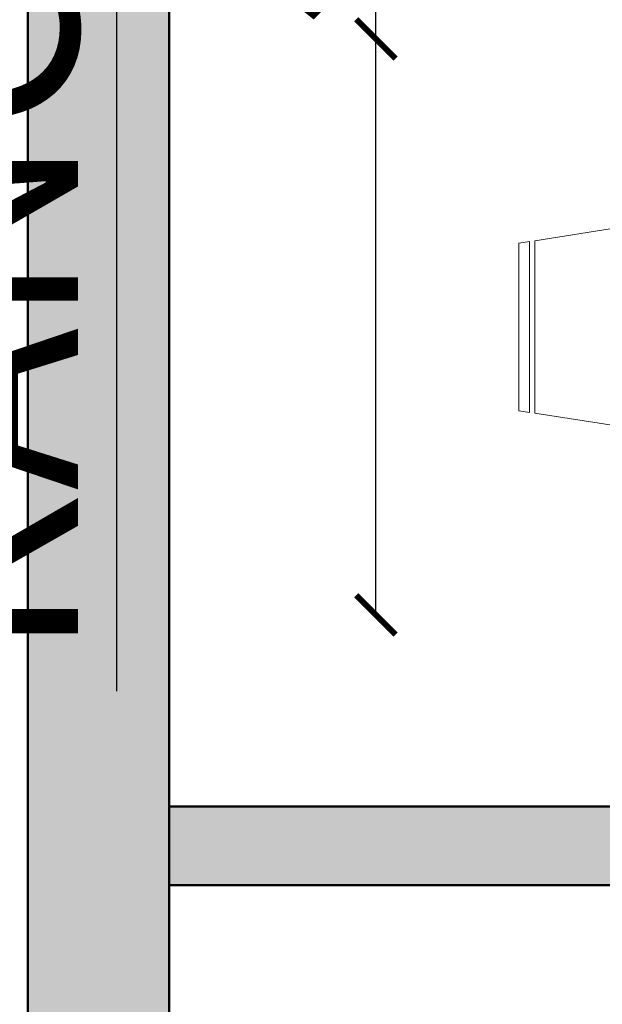
# Model space of a CAD drawing. Units: inches. Extents: x 2419 to 2878, y 1068 to 1713.
# Tile 3 of 20: x 2471 to 2508, y 1286 to 1349. Entities that reach past the tile are written whole.
import ezdxf

# ---------------------------------------------------------------- set-up
doc = ezdxf.new("R2010")
doc.units = ezdxf.units.IN
for name, color, linetype, lineweight in [('A-ANNO-DIMS', 2, 'Continuous', 18), ('A-FLOR-PRKG-PATT', 1, 'Continuous', 13), ('A-FURN', 8, 'Continuous', 18), ('A-WALL', 7, 'Continuous', 50)]:
    doc.layers.add(name, color=color, linetype=linetype, lineweight=lineweight)
doc.layers.add('A-WALL-PATT', color=18, linetype='Continuous', lineweight=13, true_color=0x000000)
doc.styles.get("Standard").update_dxf_attribs({"font": 'arial.ttf'})
doc.dimstyles.new('ISO-25', dxfattribs={"dimtxt": 12.5, "dimasz": 2.5, "dimexe": 1.25, "dimexo": 0.625, "dimtad": 1, "dimdec": 0, "dimlunit": 4, "dimtxsty": 'Standard', "dimblk": 'ARCHTICK', "dimcen": 2.5, "dimse1": 1, "dimse2": 1, "dimclrd": 4, "dimadec": 0, "dimazin": 0, "dimtfac": 1, "dimtdec": 0, "dimtmove": 0, "dimatfit": 3, "dimfxl": 1, "dimarcsym": 0})

# ---------------------------------------------------------------- blocks, each defined once
blk = doc.blocks.new('Dining Set - 36 x 72 in.')
for p, q in [((-22, 27.5), (-22.1562, 26.50042)), ((-22, 27.5), (-6, 27.5)), ((-5.8437, 26.49966), (-6, 27.5)), ((6, 27.5), (5.8438, 26.50042)), ((6, 27.5), (22, 27.5)), ((22.1563, 26.49966), (22, 27.5)), ((-5.8416, 26.5), (-22.1534, 26.5)), ((22.1584, 26.5), (5.8466, 26.5)), ((-22.2343, 26.00059), (-23.4847, 17.99762)), ((-22.2304, 26), (-5.7608, 26)), ((-4.5152, 17.99762), (-5.7655, 25.99926)), ((5.7657, 26.00059), (4.5153, 17.99762)), ((5.7696, 26), (22.2392, 26)), ((23.4848, 17.99762), (22.2345, 25.99926)), ((36, 18), (-36, 18)), ((-36, 18), (-36, -18)), ((36, -18), (36, 18)), ((-44.0006, 8.23428), (-35.9976, 9.48474)), ((44.0006, 8.23428), (35.9976, 9.48474)), ((-45.5, 8), (-44.5004, 8.15617)), ((-45.5, 8), (-45.5, -8)), ((-44.5, -8.15843), (-44.5, 8.15338)), ((-44, 8.23041), (-44, -8.23915)), ((44, 8.23041), (44, -8.23915)), ((44.5, -8.15843), (44.5, 8.15338)), ((45.5, 8), (44.5005, 8.15617)), ((45.5, 8), (45.5, -8)), ((-44.4997, -8.15631), (-45.5, -8)), ((-35.9976, -9.48476), (-43.9993, -8.2345)), ((35.9976, -9.48476), (43.9993, -8.2345)), ((44.4997, -8.15631), (45.5, -8)), ((-36, -18), (36, -18)), ((-22.2343, -26.0006), (-23.4847, -17.99762)), ((-4.5152, -17.99762), (-5.7655, -25.99928)), ((5.7657, -26.0006), (4.5153, -17.99762)), ((23.4848, -17.99762), (22.2345, -25.99928)), ((-22.2304, -26), (-5.7608, -26)), ((5.7696, -26), (22.2392, -26)), ((-22, -27.5), (-22.1562, -26.50044)), ((-5.8416, -26.5), (-22.1534, -26.5)), ((-5.8437, -26.49967), (-6, -27.5)), ((6, -27.5), (5.8438, -26.50044)), ((22.1584, -26.5), (5.8466, -26.5)), ((22.1563, -26.49967), (22, -27.5)), ((-22, -27.5), (-6, -27.5)), ((6, -27.5), (22, -27.5))]:
    blk.add_line(p, q)
for points in [[(-36, 15), (-31.1772, 14.97754), (-26.8079, 14.91406), (-22.8538, 14.81543), (-19.276, 14.6875), (-16.0362, 14.53613), (-13.0957, 14.36718), (-10.4159, 14.18652), (-7.9583, 14), (-5.6904, 13.81315), (-3.6035, 13.63021), (-1.6954, 13.45508), (0.0365, 13.29166), (1.5945, 13.14388), (2.9811, 13.01562), (4.1988, 12.9108), (5.25, 12.83333), (6.1393, 12.78613), (6.8802, 12.76823), (7.4883, 12.77767), (7.9792, 12.8125), (8.3685, 12.87077), (8.6719, 12.95052), (8.9049, 13.0498), (9.0833, 13.16666), (9.2205, 13.29899), (9.3216, 13.44401), (9.3895, 13.59879), (9.4271, 13.76041), (9.4373, 13.92594), (9.4232, 14.09245), (9.3875, 14.257), (9.3333, 14.41666), (9.2638, 14.56917), (9.1836, 14.71484), (9.0975, 14.85465), (9.0104, 14.98958), (8.9272, 15.1206), (8.8529, 15.2487), (8.7922, 15.37483), (8.75, 15.5), (8.7305, 15.62467), (8.7344, 15.74739), (8.7617, 15.86621), (8.8125, 15.97916), (8.8867, 16.08431), (8.9844, 16.17968), (9.1055, 16.26334), (9.25, 16.33333), (9.4189, 16.38802), (9.6172, 16.42708), (9.8506, 16.45052), (10.125, 16.45833), (10.4463, 16.45052), (10.8203, 16.42708), (11.2529, 16.38802), (11.75, 16.33333), (12.3184, 16.26318), (12.9694, 16.17838), (13.7151, 16.07991), (14.5677, 15.96875), (15.5395, 15.84586), (16.6426, 15.71224), (17.8893, 15.56884), (19.2917, 15.41666), (20.859, 15.25667), (22.5879, 15.08984), (24.4721, 14.91715), (26.5052, 14.73958), (28.6809, 14.5581), (30.9929, 14.3737), (33.4347, 14.18733), (36, 14)], [(-36, 10), (-28.9766, 10.14274), (-23.1725, 10.20442), (-18.4241, 10.19775), (-14.5677, 10.13541), (-11.4399, 10.03011), (-8.877, 9.89453), (-6.7154, 9.74137), (-4.7917, 9.58333), (-2.9698, 9.43082), (-1.2246, 9.28515), (0.4415, 9.14534), (2.026, 9.01041), (3.5266, 8.87939), (4.9408, 8.7513), (6.266, 8.62516), (7.5, 8.5), (8.6411, 8.37549), (9.6914, 8.2539), (10.6538, 8.13818), (11.5312, 8.03125), (12.3267, 7.93603), (13.043, 7.85547), (13.6831, 7.79248), (14.25, 7.75), (14.7471, 7.7303), (15.1797, 7.73307), (15.5537, 7.75732), (15.875, 7.80208), (16.1494, 7.86637), (16.3828, 7.94922), (16.5811, 8.04964), (16.75, 8.16666), (16.8944, 8.29915), (17.0143, 8.44531), (17.1089, 8.60319), (17.1771, 8.77083), (17.218, 8.94629), (17.2305, 9.1276), (17.2137, 9.31282), (17.1667, 9.5), (17.0895, 9.6875), (16.987, 9.875), (16.8649, 10.0625), (16.7292, 10.25), (16.5856, 10.4375), (16.4401, 10.625), (16.2985, 10.8125), (16.1667, 11), (16.05, 11.18733), (15.9518, 11.3737), (15.8752, 11.5581), (15.8229, 11.73958), (15.798, 11.91715), (15.8034, 12.08984), (15.842, 12.25667), (15.9167, 12.41666), (16.0295, 12.56836), (16.1784, 12.70833), (16.3605, 12.83268), (16.5729, 12.9375), (16.8127, 13.01888), (17.0768, 13.07291), (17.3625, 13.0957), (17.6667, 13.08333), (17.9894, 13.03312), (18.3418, 12.94726), (18.7382, 12.82918), (19.1927, 12.68229), (19.7195, 12.51001), (20.3327, 12.31575), (21.0465, 12.10294), (21.875, 11.875), (22.8357, 11.63354), (23.959, 11.37304), (25.2786, 11.08618), (26.8282, 10.76562), (28.6414, 10.40405), (30.752, 9.99414), (33.1936, 9.52856), (36, 9)], [(-36, 5.5), (-30.7157, 5.3348), (-26.069, 5.20963), (-21.9946, 5.11767), (-18.4271, 5.05208), (-15.3009, 5.00602), (-12.5508, 4.97265), (-10.1112, 4.94515), (-7.9167, 4.91666), (-5.909, 4.88167), (-4.0586, 4.83984), (-2.3429, 4.79215), (-0.7396, 4.73958), (0.7739, 4.6831), (2.22, 4.6237), (3.6213, 4.56233), (5, 4.5), (6.373, 4.43782), (7.7344, 4.3776), (9.0723, 4.32129), (10.375, 4.27083), (11.6309, 4.22819), (12.8281, 4.19531), (13.9551, 4.17415), (15, 4.16666), (15.954, 4.17448), (16.819, 4.19791), (17.6001, 4.23698), (18.3021, 4.29166), (18.9299, 4.36198), (19.4883, 4.44791), (19.9823, 4.54948), (20.4167, 4.66666), (20.7969, 4.79899), (21.1302, 4.94401), (21.4245, 5.09879), (21.6875, 5.26041), (21.9271, 5.42594), (22.1511, 5.59245), (22.3672, 5.757), (22.5834, 5.91666), (22.8065, 6.06868), (23.0404, 6.21093), (23.2879, 6.34147), (23.5521, 6.45833), (23.8358, 6.55957), (24.142, 6.64323), (24.4735, 6.70735), (24.8334, 6.75), (25.2235, 6.76969), (25.642, 6.76692), (26.0858, 6.74267), (26.5521, 6.69791), (27.0379, 6.63362), (27.5404, 6.55078), (28.0565, 6.45036), (28.5834, 6.33333), (29.1242, 6.19987), (29.7071, 6.04687), (30.3661, 5.87044), (31.1354, 5.66666), (32.0493, 5.43164), (33.142, 5.16146), (34.4475, 4.85221), (36, 4.5)], [(-36, -1), (-30.7915, -0.6591), (-26.0195, -0.38216), (-21.6519, -0.16284), (-17.6563, 0.00521), (-14.0005, 0.12833), (-10.6523, 0.21289), (-7.5796, 0.26522), (-4.75, 0.29166), (-2.134, 0.29793), (0.2878, 0.28711), (2.5317, 0.26163), (4.6146, 0.22396), (6.5529, 0.17651), (8.3633, 0.12174), (10.0623, 0.06209), (11.6667, 0), (13.1899, -0.06201), (14.6341, -0.1211), (15.9982, -0.17432), (17.2813, -0.21875), (18.4823, -0.25147), (19.6003, -0.26953), (20.6343, -0.27002), (21.5834, -0.25), (22.4481, -0.20768), (23.2357, -0.14584), (23.9549, -0.06836), (24.6146, 0.02083), (25.2235, 0.11784), (25.7904, 0.21875), (26.3241, 0.31966), (26.8334, 0.41666), (27.3265, 0.50618), (27.8099, 0.58593), (28.2894, 0.65397), (28.7709, 0.70833), (29.2601, 0.74707), (29.763, 0.76823), (30.2855, 0.76985), (30.8334, 0.75), (31.4088, 0.70784), (31.9994, 0.64713), (32.589, 0.57275), (33.1615, 0.48958), (33.7008, 0.4025), (34.1908, 0.3164), (34.6153, 0.23616), (34.9584, 0.16666), (35.2099, 0.11165), (35.3848, 0.07031), (35.504, 0.04069), (35.5886, 0.02083), (35.6594, 0.00879), (35.7377, 0.0026), (35.8442, 0.00032), (36, 0)], [(-36, -6.5), (-27.1843, -6.31267), (-20.084, -6.1263), (-14.469, -5.9419), (-10.1094, -5.76042), (-6.7752, -5.58285), (-4.2363, -5.41016), (-2.2629, -5.24333), (-0.625, -5.08334), (0.8708, -4.93099), (2.2715, -4.78646), (3.5872, -4.64974), (4.8281, -4.52084), (6.0046, -4.39974), (7.127, -4.28646), (8.2053, -4.18099), (9.25, -4.08334), (10.2705, -3.99382), (11.2734, -3.91407), (12.2647, -3.84603), (13.25, -3.79167), (14.2354, -3.75293), (15.2266, -3.73177), (16.2295, -3.73015), (17.25, -3.75), (18.2912, -3.79248), (19.3451, -3.85547), (20.4009, -3.93604), (21.4479, -4.03125), (22.4754, -4.13819), (23.4727, -4.25391), (24.4289, -4.37549), (25.3334, -4.5), (26.1785, -4.62492), (26.9694, -4.74935), (27.7145, -4.87281), (28.4219, -4.99479), (29.1, -5.11483), (29.7572, -5.23242), (30.4016, -5.34709), (31.0417, -5.45834), (31.6837, -5.56437), (32.3262, -5.65821), (32.9658, -5.73153), (33.599, -5.77604), (34.2224, -5.78345), (34.8327, -5.74545), (35.4264, -5.65373), (36, -5.5)], [(-36, -10), (-26.4022, -9.81299), (-18.4675, -9.62891), (-11.9839, -9.45069), (-6.7396, -9.28125), (-2.5226, -9.12354), (0.8789, -8.98047), (3.6769, -8.85498), (6.0833, -8.75), (8.2767, -8.66765), (10.3021, -8.60677), (12.1712, -8.56543), (13.8958, -8.54167), (15.4876, -8.53353), (16.9583, -8.53907), (18.3197, -8.55632), (19.5834, -8.58334), (20.7616, -8.61841), (21.8685, -8.66081), (22.9188, -8.71004), (23.9271, -8.76563), (24.9081, -8.82707), (25.8763, -8.89388), (26.8465, -8.96558), (27.8334, -9.04167), (28.8474, -9.12118), (29.8828, -9.20117), (30.93, -9.27824), (31.9792, -9.34896), (33.0205, -9.40991), (34.0443, -9.45768), (35.0407, -9.48885), (36, -9.5)], [(-36, -14.5), (-30.0881, -14.33513), (-25.0332, -14.21224), (-20.7312, -14.12647), (-17.0781, -14.07292), (-13.97, -14.04671), (-11.3027, -14.04297), (-8.9724, -14.05681), (-6.875, -14.08334), (-4.9224, -14.11833), (-3.0905, -14.16016), (-1.3709, -14.20785), (0.2448, -14.26042), (1.7647, -14.3169), (3.1973, -14.3763), (4.5507, -14.43767), (5.8333, -14.5), (7.0554, -14.5621), (8.235, -14.62175), (9.3922, -14.67652), (10.5469, -14.72396), (11.7192, -14.76164), (12.929, -14.78711), (14.1965, -14.79794), (15.5417, -14.79167), (16.9933, -14.76424), (18.6152, -14.70508), (20.4804, -14.60197), (22.6615, -14.44271), (25.2312, -14.21509), (28.2624, -13.9069), (31.8277, -13.50594), (36, -13)]]:
    blk.add_lwpolyline(points)
blk = doc.blocks.new('_ArchTick')
at = {"color": 0, "linetype": 'ByBlock', "const_width": 0.15}
blk.add_lwpolyline([(-0.5, -0.5), (0.5, 0.5)], dxfattribs=at)
blk = doc.blocks.new('*D26')
at = {"layer": 'A-ANNO-DIMS', "color": 4, "lineweight": -2, "transparency": 16777216}
for p, q in [((2502.769, 1356.79), (2563.458, 1356.79)), ((2563.458, 1356.79), (2733.724, 1356.79))]:
    blk.add_line(p, q, dxfattribs=at)
at = {"layer": 'Defpoints', "color": 0, "transparency": 16777216}
for p in [(2563.458, 1356.79), (2502.769, 1347.687), (2563.458, 1347.687)]:
    blk.add_point(p, dxfattribs=at)
at = {"layer": 'A-ANNO-DIMS', "color": 4, "lineweight": -2, "transparency": 16777216, "xscale": 2.5, "yscale": 2.5, "zscale": 2.5, "rotation": 180}
blk.add_blockref('_ArchTick', (2502.769, 1356.79), dxfattribs=at)
at = {"layer": 'A-ANNO-DIMS', "color": 4, "lineweight": -2, "transparency": 16777216, "xscale": 2.5, "yscale": 2.5, "zscale": 2.5}
blk.add_blockref('_ArchTick', (2563.458, 1356.79), dxfattribs=at)
at = {"layer": 'A-ANNO-DIMS', "color": 0, "transparency": 16777216, "insert": (2649.841, 1363.878), "char_height": 12.5, "attachment_point": 5}
blk.add_mtext('DINING SET 5\'-0 1/2"', dxfattribs=at)
blk = doc.blocks.new('*D27')
at = {"layer": 'A-ANNO-DIMS', "color": 4, "lineweight": -2, "transparency": 16777216}
for p, q in [((2493.665, 1347.687), (2493.665, 1413.783)), ((2493.665, 1311.006), (2493.665, 1347.687))]:
    blk.add_line(p, q, dxfattribs=at)
at = {"layer": 'Defpoints', "color": 0, "transparency": 16777216}
for p in [(2493.665, 1347.687), (2502.769, 1347.687), (2502.769, 1311.006)]:
    blk.add_point(p, dxfattribs=at)
at = {"layer": 'A-ANNO-DIMS', "color": 4, "lineweight": -2, "transparency": 16777216, "xscale": 2.5, "yscale": 2.5, "zscale": 2.5}
for p, rotation in [((2493.665, 1347.687), 90), ((2493.665, 1311.006), 270)]:
    blk.add_blockref('_ArchTick', p, dxfattribs=dict(at, rotation=rotation))
at = {"layer": 'A-ANNO-DIMS', "color": 0, "transparency": 16777216, "insert": (2486.573, 1381.985), "char_height": 12.5, "attachment_point": 5, "rotation": 90}
blk.add_mtext('3\'-0 1/2"', dxfattribs=at)
blk = doc.blocks.new('*D28')
at = {"layer": 'A-ANNO-DIMS', "color": 4, "lineweight": -2, "transparency": 16777216}
for p, q in [((2477.16, 1470.633), (2477.16, 1448.272)), ((2477.16, 1448.272), (2477.16, 1306.152))]:
    blk.add_line(p, q, dxfattribs=at)
at = {"layer": 'Defpoints', "color": 0, "transparency": 16777216}
for p in [(2480.514, 1470.633), (2477.16, 1448.272), (2480.514, 1448.272)]:
    blk.add_point(p, dxfattribs=at)
at = {"layer": 'A-ANNO-DIMS', "color": 4, "lineweight": -2, "transparency": 16777216, "xscale": 2.5, "yscale": 2.5, "zscale": 2.5}
for p, rotation in [((2477.16, 1470.633), 90), ((2477.16, 1448.272), 270)]:
    blk.add_blockref('_ArchTick', p, dxfattribs=dict(at, rotation=rotation))
at = {"layer": 'A-ANNO-DIMS', "color": 0, "transparency": 16777216, "insert": (2470.072, 1375.962), "char_height": 12.5, "attachment_point": 5, "rotation": 90}
blk.add_mtext('RANGE 1\'-10 1/2"', dxfattribs=at)
blk = doc.blocks.new('*D43')
at = {"layer": 'A-ANNO-DIMS', "color": 4, "lineweight": -2, "transparency": 16777216}
blk.add_line((2480.514, 1079.925), (2557.299, 1079.925), dxfattribs=at)
at = {"layer": 'Defpoints', "color": 0, "transparency": 16777216}
for p in [(2480.514, 1408.813), (2557.299, 1408.813), (2557.299, 1079.925)]:
    blk.add_point(p, dxfattribs=at)
at = {"layer": 'A-ANNO-DIMS', "color": 4, "lineweight": -2, "transparency": 16777216, "xscale": 2.5, "yscale": 2.5, "zscale": 2.5, "rotation": 180}
blk.add_blockref('_ArchTick', (2480.514, 1079.925), dxfattribs=at)
at = {"layer": 'A-ANNO-DIMS', "color": 4, "lineweight": -2, "transparency": 16777216, "xscale": 2.5, "yscale": 2.5, "zscale": 2.5}
blk.add_blockref('_ArchTick', (2557.299, 1079.925), dxfattribs=at)
at = {"layer": 'A-ANNO-DIMS', "color": 0, "transparency": 16777216, "insert": (2518.907, 1086.932), "char_height": 12.5, "attachment_point": 5}
blk.add_mtext('6\'-5"', dxfattribs=at)
blk = doc.blocks.new('*D47')
at = {"layer": 'A-ANNO-DIMS', "color": 4, "lineweight": -2, "transparency": 16777216}
for p, q in [((2444.314, 1376.561), (2444.314, 1357.976)), ((2444.314, 1357.976), (2444.314, 1293.048))]:
    blk.add_line(p, q, dxfattribs=at)
at = {"layer": 'Defpoints', "color": 0, "transparency": 16777216}
for p in [(2632.514, 1376.561), (2444.314, 1357.976), (2632.514, 1357.976)]:
    blk.add_point(p, dxfattribs=at)
at = {"layer": 'A-ANNO-DIMS', "color": 4, "lineweight": -2, "transparency": 16777216, "xscale": 2.5, "yscale": 2.5, "zscale": 2.5}
for p, rotation in [((2444.314, 1376.561), 90), ((2444.314, 1357.976), 270)]:
    blk.add_blockref('_ArchTick', p, dxfattribs=dict(at, rotation=rotation))
at = {"layer": 'A-ANNO-DIMS', "color": 0, "transparency": 16777216, "insert": (2437.226, 1324.262), "char_height": 12.5, "attachment_point": 5, "rotation": 90}
blk.add_mtext('1\'-6 1/2"', dxfattribs=at)
blk = doc.blocks.new('*D54')
at = {"layer": 'A-ANNO-DIMS', "color": 4, "lineweight": -2, "transparency": 16777216}
blk.add_line((2444.314, 1130.813), (2444.314, 1293.813), dxfattribs=at)
at = {"layer": 'Defpoints', "color": 0, "transparency": 16777216}
for p in [(2444.314, 1293.813), (2480.514, 1293.813), (2480.514, 1130.813)]:
    blk.add_point(p, dxfattribs=at)
at = {"layer": 'A-ANNO-DIMS', "color": 4, "lineweight": -2, "transparency": 16777216, "xscale": 2.5, "yscale": 2.5, "zscale": 2.5}
for p, rotation in [((2444.314, 1293.813), 90), ((2444.314, 1130.813), 270)]:
    blk.add_blockref('_ArchTick', p, dxfattribs=dict(at, rotation=rotation))
at = {"layer": 'A-ANNO-DIMS', "color": 0, "transparency": 16777216, "insert": (2437.303, 1212.313), "char_height": 12.5, "attachment_point": 5, "rotation": 90}
blk.add_mtext('13\'-7"', dxfattribs=at)
blk = doc.blocks.new('*D56')
at = {"layer": 'A-ANNO-DIMS', "color": 4, "lineweight": -2, "transparency": 16777216}
for p, q in [((2480.514, 1079.925), (2503.967, 1079.925)), ((2503.967, 1079.925), (2578.607, 1079.925))]:
    blk.add_line(p, q, dxfattribs=at)
at = {"layer": 'Defpoints', "color": 0, "transparency": 16777216}
for p in [(2480.514, 1507.813), (2503.967, 1494.852), (2503.967, 1079.925)]:
    blk.add_point(p, dxfattribs=at)
at = {"layer": 'A-ANNO-DIMS', "color": 4, "lineweight": -2, "transparency": 16777216, "xscale": 2.5, "yscale": 2.5, "zscale": 2.5, "rotation": 180}
blk.add_blockref('_ArchTick', (2480.514, 1079.925), dxfattribs=at)
at = {"layer": 'A-ANNO-DIMS', "color": 4, "lineweight": -2, "transparency": 16777216, "xscale": 2.5, "yscale": 2.5, "zscale": 2.5}
blk.add_blockref('_ArchTick', (2503.967, 1079.925), dxfattribs=at)
at = {"layer": 'A-ANNO-DIMS', "color": 0, "transparency": 16777216, "insert": (2542.537, 1087.013), "char_height": 12.5, "attachment_point": 5}
blk.add_mtext('1\'-11 1/2"', dxfattribs=at)
blk = doc.blocks.new('*D59')
at = {"layer": 'A-ANNO-DIMS', "color": 4, "lineweight": -2, "transparency": 16777216}
blk.add_line((2480.514, 1079.925), (2589.514, 1079.925), dxfattribs=at)
at = {"layer": 'Defpoints', "color": 0, "transparency": 16777216}
for p in [(2480.514, 1414.813), (2589.514, 1414.813), (2589.514, 1079.925)]:
    blk.add_point(p, dxfattribs=at)
at = {"layer": 'A-ANNO-DIMS', "color": 4, "lineweight": -2, "transparency": 16777216, "xscale": 2.5, "yscale": 2.5, "zscale": 2.5, "rotation": 180}
blk.add_blockref('_ArchTick', (2480.514, 1079.925), dxfattribs=at)
at = {"layer": 'A-ANNO-DIMS', "color": 4, "lineweight": -2, "transparency": 16777216, "xscale": 2.5, "yscale": 2.5, "zscale": 2.5}
blk.add_blockref('_ArchTick', (2589.514, 1079.925), dxfattribs=at)
at = {"layer": 'A-ANNO-DIMS', "color": 0, "transparency": 16777216, "insert": (2535.014, 1086.932), "char_height": 12.5, "attachment_point": 5}
blk.add_mtext('9\'-1"', dxfattribs=at)

msp = doc.modelspace()

# ---------------------------------------------------------------- hatches: boundary and pattern name
at = {"layer": 'A-FLOR-PRKG-PATT'}
h = msp.add_hatch(color=256, dxfattribs=at)
h.dxf.hatch_style = 1
edge = h.paths.add_edge_path()
edge.add_ellipse((2561.374, 1279.453), major_axis=(3.988, 0), ratio=0.842304, start_angle=0.64655, end_angle=90)
edge.add_line((2561.374, 1282.813), (2511.571, 1282.813))
edge.add_ellipse((2511.571, 1279.453), major_axis=(3.988, 0), ratio=0.842304, start_angle=90, end_angle=179.35345)
edge.add_ellipse((10560.892, 1188.617), major_axis=(-8054.031, 0), ratio=0.84230387, start_angle=-0.6465541, end_angle=-0.6282372)
edge.add_ellipse((2509.23, 1276.906), major_axis=(1.687, 0), ratio=0.842304, start_angle=179.37176, end_angle=248.46476)
edge.add_ellipse((10560.329, 1188.617), major_axis=(8052.293, 0), ratio=0.84230387, start_angle=179.3534459, end_angle=179.3813568, ccw=False)
edge.add_ellipse((2511.008, 1279.453), major_axis=(2.25, 0), ratio=0.842304, start_angle=90, end_angle=179.35345, ccw=False)
edge.add_line((2511.008, 1281.348), (2561.936, 1281.348))
edge.add_ellipse((2561.936, 1279.453), major_axis=(-2.25, 0), ratio=0.842304, start_angle=180.64655, end_angle=270, ccw=False)
edge.add_ellipse((-5487.385, 1188.617), major_axis=(8052.293, 0), ratio=0.84230387, start_angle=0.5282715, end_angle=0.6465541, ccw=False)
edge.add_ellipse((2563.715, 1276.906), major_axis=(-1.687, 0), ratio=0.842304, start_angle=111.53524, end_angle=180.62824)
edge.add_ellipse((-5487.947, 1188.617), major_axis=(-8054.031, 0), ratio=0.84230387, start_angle=180.6282372, end_angle=180.6465541)
edge = h.paths.add_edge_path()
edge.add_ellipse((2564.908, 1261.91), major_axis=(-1.125, 0), ratio=0.842304, start_angle=180, end_angle=270)
edge.add_line((2564.908, 1262.857), (2564.426, 1262.857))
edge.add_ellipse((-5487.385, 1188.617), major_axis=(8052.293, 0), ratio=0.84230387, start_angle=0.3838668, end_angle=0.5282715, ccw=False)
edge.add_line((2564.654, 1242.564), (2564.908, 1242.564))
edge.add_ellipse((2564.908, 1243.512), major_axis=(-1.125, 0), ratio=0.842304, start_angle=90, end_angle=180)
edge.add_line((2566.033, 1243.512), (2566.033, 1261.91))
edge = h.paths.add_edge_path()
edge.add_ellipse((2564.908, 1174.989), major_axis=(1.125, 0), ratio=0.842304, start_angle=0, end_angle=90)
edge.add_line((2564.908, 1175.936), (2564.894, 1175.936))
edge.add_ellipse((-5487.385, 1188.617), major_axis=(8052.293, 0), ratio=0.84230387, start_angle=-0.1349866, end_angle=-0.0902291, ccw=False)
edge.add_ellipse((2163.343, 1170.913), major_axis=(401.537, 0), ratio=0.8423039, start_angle=-2.17995, end_angle=-0.13561, ccw=False)
edge.add_line((2564.47, 1155.643), (2564.908, 1155.643))
edge.add_ellipse((2564.908, 1156.591), major_axis=(-1.125, 0), ratio=0.842304, start_angle=90, end_angle=180)
edge.add_line((2566.033, 1156.591), (2566.033, 1174.989))
h.paths.add_polyline_path([(2574.476, 1207.448), (2633.94, 1207.448), (2633.94, 1217.366), (2574.476, 1217.366)], flags=9)
h.paths.add_polyline_path([(2574.454, 1217.828), (2610.472, 1217.828), (2610.472, 1227.879), (2574.454, 1227.879)], flags=9)
h.paths.add_polyline_path([(2672.426, 1304.02), (2718.617, 1304.02), (2718.617, 1313.939), (2672.426, 1313.939)], flags=9)
h.paths.add_polyline_path([(2672.404, 1314.4), (2750.128, 1314.4), (2750.128, 1324.451), (2672.404, 1324.451)], flags=9)
h.paths.add_polyline_path([(2500.432, 1374.444), (2544.803, 1374.444), (2544.803, 1384.362), (2500.432, 1384.362)], flags=9)
h.paths.add_polyline_path([(2500.41, 1384.824), (2566.075, 1384.824), (2566.075, 1394.875), (2500.41, 1394.875)], flags=9)
h.paths.add_polyline_path([(2738.933, 1376.749), (2778.273, 1376.749), (2778.273, 1386.667), (2738.933, 1386.667)], flags=9)
h.paths.add_polyline_path([(2659.12, 1357.8), (2703.492, 1357.8), (2703.492, 1367.718), (2659.12, 1367.718)], flags=9)
h.paths.add_polyline_path([(2659.098, 1368.18), (2694.114, 1368.18), (2694.114, 1378.23), (2659.098, 1378.23)], flags=9)
h.paths.add_polyline_path([(2730.123, 1466.067), (2769.463, 1466.067), (2769.463, 1475.986), (2730.123, 1475.986)], flags=9)
h.paths.add_polyline_path([(2730.101, 1476.447), (2765.117, 1476.447), (2765.117, 1486.498), (2730.101, 1486.498)], flags=9)
h.paths.add_polyline_path([(2730.382, 1518.647), (2761.48, 1518.647), (2761.48, 1528.566), (2730.382, 1528.566)], flags=9)
h.paths.add_polyline_path([(2730.361, 1529.028), (2780.958, 1529.028), (2780.958, 1539.072), (2730.361, 1539.072)], flags=9)
h.paths.add_polyline_path([(2629.32, 1455.189), (2688.784, 1455.189), (2688.784, 1465.107), (2629.32, 1465.107)], flags=9)
h.paths.add_polyline_path([(2629.298, 1465.569), (2681.902, 1465.569), (2681.902, 1475.62), (2629.298, 1475.62)], flags=9)
h.paths.add_polyline_path([(2513.229, 1456.484), (2562.631, 1456.484), (2562.631, 1466.402), (2513.229, 1466.402)], flags=9)
h.paths.add_polyline_path([(2513.208, 1466.865), (2556.26, 1466.865), (2556.26, 1476.909), (2513.208, 1476.909)], flags=9)
h.paths.add_polyline_path([(2488.87, 1521.538), (2519.968, 1521.538), (2519.968, 1531.456), (2488.87, 1531.456)], flags=9)
h.paths.add_polyline_path([(2536.549, 1543.507), (2580.923, 1543.507), (2580.923, 1553.432), (2536.549, 1553.432)], flags=9)
h.paths.add_polyline_path([(2536.557, 1553.921), (2573.525, 1553.921), (2573.525, 1563.8), (2536.557, 1563.8)], flags=9)
at = {"layer": 'A-WALL-PATT'}
h = msp.add_hatch(color=256, dxfattribs=at)
h.dxf.hatch_style = 1
h.paths.add_polyline_path([(2780.514, 1577.813), (2471.514, 1577.813), (2471.514, 1121.813), (2780.514, 1121.813)])
h.paths.add_polyline_path([(2480.514, 1568.813), (2771.514, 1568.813), (2771.514, 1130.813), (2480.514, 1130.813)], flags=16)
h.paths.add_polyline_path([(2528.514, 1568.813), (2528.514, 1512.813), (2594.514, 1512.813), (2594.514, 1414.813), (2596.568, 1414.813), (2596.568, 1441.609), (2597.816, 1441.609), (2597.816, 1441.582, -0.384016), (2625.035, 1414.813), (2725.514, 1414.813), (2725.514, 1567.545), (2728.302, 1567.545), (2746.887, 1567.545), (2746.887, 1566.732), (2746.87, 1566.732, -0.367216), (2730.514, 1549.092), (2730.514, 1512.813), (2750.853, 1512.813), (2750.853, 1510.025, -0.401453), (2733.081, 1491.458), (2733.081, 1491.44), (2732.268, 1491.44), (2732.268, 1507.813), (2730.514, 1507.813), (2730.514, 1408.813), (2736.514, 1408.813), (2736.514, 1349.813), (2632.514, 1349.813), (2632.514, 1408.813), (2528.514, 1408.813), (2528.514, 1414.813), (2503.967, 1414.813), (2503.967, 1494.852), (2558.379, 1494.852), (2558.379, 1507.813), (2529.965, 1507.813, -0.414214), (2530.821, 1506.957), (2530.821, 1497.257, -0.414214), (2529.965, 1496.401), (2514.559, 1496.401, -0.414214), (2513.703, 1497.257), (2513.703, 1506.957, -0.414214), (2514.559, 1507.813), (2528.514, 1507.813), (2528.514, 1512.813), (2480.514, 1512.813)], flags=0)
h.paths.add_polyline_path([(2516.262, 1507.813), (2528.262, 1507.813), (2528.262, 1505.813), (2523.417, 1505.813), (2524.074, 1504.675), (2529.394, 1504.675, -0.414214), (2529.965, 1504.104), (2529.965, 1497.828, -0.414214), (2529.394, 1497.257), (2515.13, 1497.257, -0.414214), (2514.559, 1497.828), (2514.559, 1504.104, -0.414214), (2515.13, 1504.675), (2520.689, 1504.675), (2521.342, 1505.813), (2516.262, 1505.813)], flags=0)
h.paths.add_polyline_path([(2522.016, 1505.531), (2522.817, 1507.318, -0.65506), (2522.254, 1506.063), (2522.195, 1505.93), (2522.425, 1505.531)], flags=0)
h.paths.add_polyline_path([(2522.833, 1500.966, -1), (2521.691, 1500.966, -1)], flags=0)
h.paths.add_polyline_path([(2522.547, 1500.966, -1), (2521.977, 1500.966, -1)], flags=0)
h.paths.add_polyline_path([(2482.005, 1470.633), (2499.894, 1470.633), (2499.894, 1448.272), (2482.005, 1448.272), (2482.005, 1452.744), (2481.26, 1452.744), (2481.26, 1449.763), (2480.514, 1449.763), (2480.514, 1469.142), (2481.26, 1469.142), (2481.26, 1466.16), (2482.005, 1466.16)], flags=0)
h.paths.add_polyline_path([(2488.713, 1466.16, -1), (2484.241, 1466.16, -1)], flags=0)
h.paths.add_polyline_path([(2496.167, 1466.16, -1), (2490.204, 1466.16, -1)], flags=0)
h.paths.add_polyline_path([(2487.968, 1466.16, -1), (2484.987, 1466.16, -1)], flags=0)
h.paths.add_polyline_path([(2495.422, 1466.16, -1), (2490.949, 1466.16, -1)], flags=0)
h.paths.add_polyline_path([(2487.223, 1466.16, -1), (2485.732, 1466.16, -1)], flags=0)
h.paths.add_polyline_path([(2494.676, 1466.16, -1), (2491.695, 1466.16, -1)], flags=0)
h.paths.add_polyline_path([(2499.108, 1468.005, -1), (2497.977, 1468.005, -1)], flags=0)
h.paths.add_polyline_path([(2493.931, 1466.16, -1), (2492.44, 1466.16, -1)], flags=0)
h.paths.add_polyline_path([(2499.372, 1463.71, -1), (2498.166, 1463.71, -1)], flags=0)
h.paths.add_polyline_path([(2484.241, 1461.688), (2496.167, 1461.688), (2496.167, 1457.216), (2484.241, 1457.216)], flags=0)
h.paths.add_polyline_path([(2484.987, 1460.943), (2495.422, 1460.943), (2495.422, 1457.961), (2484.987, 1457.961)], flags=0)
h.paths.add_polyline_path([(2586.88, 1510.025), (2587.693, 1510.025), (2587.693, 1491.44), (2586.88, 1491.44)], flags=0)
h.paths.add_polyline_path([(2499.259, 1459.415, -1), (2498.203, 1459.415, -1)], flags=0)
h.paths.add_polyline_path([(2489.459, 1452.744, -1), (2483.496, 1452.744, -1)], flags=0)
h.paths.add_polyline_path([(2557.299, 1408.813), (2557.299, 1413.091, -0.401453), (2584.57, 1441.582), (2584.57, 1441.609), (2585.818, 1441.609), (2585.818, 1413.091), (2585.818, 1408.813)], flags=0)
h.paths.add_polyline_path([(2488.713, 1452.744, -1), (2484.241, 1452.744, -1)], flags=0)
h.paths.add_polyline_path([(2495.422, 1452.744, -1), (2490.949, 1452.744, -1)], flags=0)
h.paths.add_polyline_path([(2487.968, 1452.744, -1), (2484.987, 1452.744, -1)], flags=0)
h.paths.add_polyline_path([(2494.676, 1452.744, -1), (2491.695, 1452.744, -1)], flags=0)
h.paths.add_polyline_path([(2487.223, 1452.744, -1), (2485.732, 1452.744, -1)], flags=0)
h.paths.add_polyline_path([(2499.183, 1454.442, -1), (2497.902, 1454.442, -1)], flags=0)
h.paths.add_polyline_path([(2493.931, 1452.744, -1), (2492.44, 1452.744, -1)], flags=0)
h.paths.add_polyline_path([(2499.296, 1450.637, -1), (2497.789, 1450.637, -1)], flags=0)
h.paths.add_polyline_path([(2619.129, 1558.889, -1), (2605.129, 1558.889, -1)], flags=0)
h.paths.add_polyline_path([(2609.129, 1558.889), (2612.129, 1561.889), (2615.129, 1558.889), (2612.129, 1555.889)], flags=0)
h.paths.add_polyline_path([(2611.129, 1558.889, -1), (2613.129, 1558.889, -1)], flags=0)
h.paths.add_polyline_path([(2633.679, 1568.813), (2693.679, 1568.813), (2693.679, 1488.813), (2633.679, 1488.813)], flags=0)
h.paths.add_polyline_path([(2641.679, 1554.413), (2641.679, 1567.613), (2662.479, 1567.613), (2662.479, 1554.413), (2664.879, 1554.413), (2664.879, 1567.613), (2685.679, 1567.613), (2685.679, 1552.413), (2680.479, 1552.413), (2693.679, 1539.213), (2678.479, 1539.213), (2678.479, 1554.413)], flags=0)
h.paths.add_polyline_path([(2637.514, 1408.813), (2731.514, 1408.813), (2731.514, 1354.813), (2637.514, 1354.813), (2637.514, 1357.976), (2635.302, 1357.976), (2635.302, 1358.789), (2637.514, 1358.789)], flags=0)
h.paths.add_polyline_path([(2717.171, 1559.643, -1), (2703.171, 1559.643, -1)], flags=0)
h.paths.add_polyline_path([(2707.171, 1559.643), (2710.171, 1562.643), (2713.171, 1559.643), (2710.171, 1556.643)], flags=0)
h.paths.add_polyline_path([(2709.171, 1559.643, -1), (2711.171, 1559.643, -1)], flags=0)
h.paths.add_polyline_path([(2685.378, 1408.813), (2706.378, 1408.813), (2706.378, 1400.813), (2699.878, 1400.813), (2701.878, 1394.813, -0.501323), (2696.923, 1375.952, -0.132891), (2694.834, 1375.952, -0.501317), (2689.878, 1394.813), (2691.878, 1400.813), (2688.878, 1400.813), (2688.878, 1399.313), (2685.878, 1399.313), (2685.878, 1400.313), (2687.878, 1400.313), (2687.878, 1400.813), (2685.378, 1400.813)], flags=0)
h.paths.add_polyline_path([(2687.378, 1407.813), (2704.378, 1407.813, -0.5), (2705.378, 1406.813), (2705.378, 1402.813, -0.5), (2704.378, 1401.813), (2687.378, 1401.813, -0.5), (2686.378, 1402.813), (2686.378, 1406.813, -0.5)], flags=0)
h.paths.add_polyline_path([(2639.514, 1205.813), (2634.514, 1205.813), (2634.514, 1293.813), (2637.514, 1293.813), (2639.514, 1293.813)], flags=0)
h.paths.add_polyline_path([(2691.878, 1394.813), (2699.878, 1394.813, -0.48008), (2697.522, 1377.29, -0.215004), (2694.234, 1377.29, -0.48008)], flags=0)
h.paths.add_polyline_path([(2757.514, 1453.891), (2763.514, 1451.891), (2763.514, 1454.891), (2762.014, 1454.891), (2762.014, 1457.891), (2763.014, 1457.891), (2763.014, 1455.891), (2763.514, 1455.891), (2763.514, 1458.391), (2771.514, 1458.391), (2771.514, 1437.391), (2763.514, 1437.391), (2763.514, 1443.891), (2757.515, 1441.891, -0.501323), (2738.653, 1446.847, -0.132891), (2738.653, 1448.936, -0.501317)], flags=0)
h.paths.add_polyline_path([(2739.991, 1449.535, -0.48008), (2757.514, 1451.891), (2757.514, 1443.891, -0.48008), (2739.991, 1446.247, -0.215004)], flags=0)
h.paths.add_polyline_path([(2765.514, 1457.391), (2769.514, 1457.391, -0.5), (2770.514, 1456.391), (2770.514, 1439.391, -0.5), (2769.514, 1438.391), (2765.514, 1438.391, -0.5), (2764.514, 1439.391), (2764.514, 1456.391, -0.5)], flags=0)
h = msp.add_hatch(color=256, dxfattribs=at)
h.dxf.hatch_style = 1
h.paths.add_polyline_path([(2771.514, 1354.813), (2736.514, 1354.813), (2736.514, 1408.813), (2771.514, 1408.813), (2771.514, 1414.813), (2625.035, 1414.813, -0.015108), (2625.087, 1413.091), (2625.087, 1408.813), (2632.514, 1408.813), (2632.514, 1376.561), (2635.302, 1376.561, -0.029838), (2637.514, 1376.429), (2637.514, 1408.813), (2731.514, 1408.813), (2731.514, 1354.813), (2637.514, 1354.813), (2637.514, 1357.976), (2635.302, 1357.976), (2632.514, 1357.976), (2632.514, 1349.813), (2771.514, 1349.813)])
h.paths.add_polyline_path([(2639.514, 1298.813), (2637.514, 1298.813), (2480.514, 1298.813), (2480.514, 1293.813), (2637.514, 1293.813), (2639.514, 1293.813)])
h.paths.add_polyline_path([(2639.514, 1293.813), (2637.514, 1293.813), (2634.514, 1293.813), (2634.514, 1244.653), (2638.792, 1244.653, -0.006332), (2639.514, 1244.644)])
h.paths.add_polyline_path([(2639.514, 1205.813), (2771.514, 1205.813), (2771.514, 1210.813), (2639.514, 1210.813), (2639.514, 1216.134), (2638.792, 1216.134), (2634.514, 1216.134), (2634.514, 1130.813), (2639.514, 1130.813)])
h.paths.add_polyline_path([(2596.568, 1413.091), (2596.568, 1414.813), (2585.818, 1414.813), (2585.818, 1413.091), (2585.818, 1408.813), (2596.568, 1408.813)])
h.paths.add_polyline_path([(2557.299, 1413.091, -0.015108), (2557.351, 1414.813), (2480.514, 1414.813), (2480.514, 1408.813), (2557.299, 1408.813)])
h.paths.add_polyline_path([(2574.476, 1207.448), (2633.94, 1207.448), (2633.94, 1217.366), (2574.476, 1217.366)], flags=9)
h.paths.add_polyline_path([(2574.454, 1217.828), (2610.472, 1217.828), (2610.472, 1227.879), (2574.454, 1227.879)], flags=9)
h.paths.add_polyline_path([(2672.426, 1304.02), (2718.617, 1304.02), (2718.617, 1313.939), (2672.426, 1313.939)], flags=9)
h.paths.add_polyline_path([(2672.404, 1314.4), (2750.128, 1314.4), (2750.128, 1324.451), (2672.404, 1324.451)], flags=9)
h.paths.add_polyline_path([(2500.432, 1374.444), (2544.803, 1374.444), (2544.803, 1384.362), (2500.432, 1384.362)], flags=9)
h.paths.add_polyline_path([(2500.41, 1384.824), (2566.075, 1384.824), (2566.075, 1394.875), (2500.41, 1394.875)], flags=9)
h.paths.add_polyline_path([(2738.933, 1376.749), (2778.273, 1376.749), (2778.273, 1386.667), (2738.933, 1386.667)], flags=9)
h.paths.add_polyline_path([(2659.12, 1357.8), (2703.492, 1357.8), (2703.492, 1367.718), (2659.12, 1367.718)], flags=25)
h.paths.add_polyline_path([(2659.098, 1368.18), (2694.114, 1368.18), (2694.114, 1378.23), (2659.098, 1378.23)], flags=25)
h.paths.add_polyline_path([(2730.123, 1466.067), (2769.463, 1466.067), (2769.463, 1475.986), (2730.123, 1475.986)], flags=9)
h.paths.add_polyline_path([(2730.101, 1476.447), (2765.117, 1476.447), (2765.117, 1486.498), (2730.101, 1486.498)], flags=9)
h.paths.add_polyline_path([(2730.382, 1518.647), (2761.48, 1518.647), (2761.48, 1528.566), (2730.382, 1528.566)], flags=9)
h.paths.add_polyline_path([(2730.361, 1529.028), (2780.958, 1529.028), (2780.958, 1539.072), (2730.361, 1539.072)], flags=9)
h.paths.add_polyline_path([(2629.32, 1455.189), (2688.784, 1455.189), (2688.784, 1465.107), (2629.32, 1465.107)], flags=9)
h.paths.add_polyline_path([(2629.298, 1465.569), (2681.902, 1465.569), (2681.902, 1475.62), (2629.298, 1475.62)], flags=9)
h.paths.add_polyline_path([(2513.229, 1456.484), (2562.631, 1456.484), (2562.631, 1466.402), (2513.229, 1466.402)], flags=9)
h.paths.add_polyline_path([(2513.208, 1466.865), (2556.26, 1466.865), (2556.26, 1476.909), (2513.208, 1476.909)], flags=9)
h.paths.add_polyline_path([(2488.87, 1521.538), (2519.968, 1521.538), (2519.968, 1531.456), (2488.87, 1531.456)], flags=9)
h.paths.add_polyline_path([(2536.549, 1543.507), (2580.923, 1543.507), (2580.923, 1553.432), (2536.549, 1553.432)], flags=9)
h.paths.add_polyline_path([(2536.557, 1553.921), (2573.525, 1553.921), (2573.525, 1563.8), (2536.557, 1563.8)], flags=9)

# ---------------------------------------------------------------- linework, layer by layer
at = {"layer": 'A-WALL'}
for p, q in [((2480.514, 1130.813), (2480.514, 1568.813)), ((2480.514, 1298.813), (2637.514, 1298.813)), ((2480.514, 1293.813), (2637.514, 1293.813))]:
    msp.add_line(p, q, dxfattribs=at)
msp.add_lwpolyline([(2471.514, 1577.813), (2780.514, 1577.813), (2780.514, 1121.813), (2471.514, 1121.813)], close=True, dxfattribs=at)

# ---------------------------------------------------------------- block references
at = {"layer": 'A-FURN', "xscale": 0.6669202688727635, "yscale": 0.6669202688727635, "zscale": 0.6669202688727635}
msp.add_blockref('Dining Set - 36 x 72 in.', (2533.113, 1329.346), dxfattribs=at)

# ---------------------------------------------------------------- dimensions: what is measured, and where the dimension line sits
at = {"layer": 'A-ANNO-DIMS'}
for base, p1, p2, picture, middle in [((2503.967, 1079.925), (2480.514, 1507.813), (2503.967, 1494.852), '*D56', (2542.537, 1087.013)), ((2589.514, 1079.925), (2480.514, 1414.813), (2589.514, 1414.813), '*D59', (2535.014, 1086.932)), ((2557.299, 1079.925), (2480.514, 1408.813), (2557.299, 1408.813), '*D43', (2518.907, 1086.932))]:
    dim = msp.add_linear_dim(base=base, p1=p1, p2=p2, dimstyle='ISO-25', override={"dimdec": 1, "dimlfac": 1, "dimrnd": 0, "dimzin": 1, "dimdsep": 46, "dimlunit": 4, "dimfrac": 2}, dxfattribs=at)
    dim.commit()
    dim.dimension.update_dxf_attribs({"geometry": picture, "text_midpoint": middle})
dim = msp.add_linear_dim(base=(2477.16, 1448.272), p1=(2480.514, 1470.633), p2=(2480.514, 1448.272), angle=270, text='RANGE <>', dimstyle='ISO-25', override={"dimdec": 1, "dimlfac": 1, "dimrnd": 0, "dimzin": 1, "dimdsep": 46, "dimlunit": 4, "dimfrac": 2}, dxfattribs=at)
dim.commit()
dim.dimension.update_dxf_attribs({"geometry": '*D28', "text_midpoint": (2470.072, 1375.962)})
for base, p1, p2, picture, middle in [((2493.665, 1347.687), (2502.769, 1311.006), (2502.769, 1347.687), '*D27', (2486.573, 1381.985)), ((2444.314, 1357.976), (2632.514, 1376.561), (2632.514, 1357.976), '*D47', (2437.226, 1324.262)), ((2444.314, 1293.813), (2480.514, 1130.813), (2480.514, 1293.813), '*D54', (2437.303, 1212.313))]:
    dim = msp.add_linear_dim(base=base, p1=p1, p2=p2, angle=90, dimstyle='ISO-25', override={"dimdec": 1, "dimlfac": 1, "dimrnd": 0, "dimzin": 1, "dimdsep": 46, "dimlunit": 4, "dimfrac": 2}, dxfattribs=at)
    dim.commit()
    dim.dimension.update_dxf_attribs({"geometry": picture, "text_midpoint": middle})
dim = msp.add_linear_dim(base=(2563.458, 1356.79), p1=(2502.769, 1347.687), p2=(2563.458, 1347.687), text='DINING SET <>', dimstyle='ISO-25', override={"dimdec": 1, "dimlfac": 1, "dimrnd": 0, "dimzin": 1, "dimdsep": 46, "dimlunit": 4, "dimfrac": 2}, dxfattribs=at)
dim.commit()
dim.dimension.update_dxf_attribs({"geometry": '*D26', "text_midpoint": (2649.841, 1363.878)})

doc.saveas('drawing.dxf')
